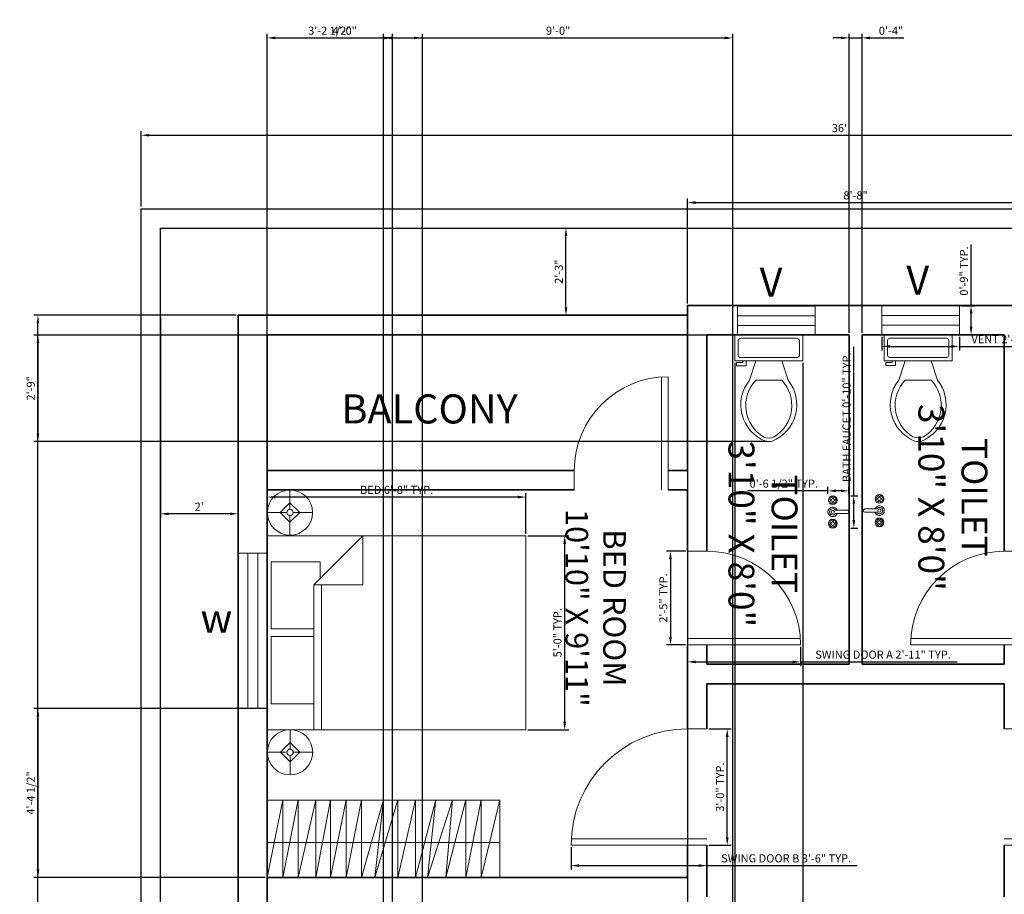
# Model space of a CAD drawing. Units: inches. Extents: x 1879 to 2382, y 1769 to 2461.
# Tile 4 of 5: x 1879 to 2183, y 2190 to 2461. Entities that reach past the tile are written whole.
import ezdxf

# ---------------------------------------------------------------- set-up
doc = ezdxf.new("R2010")
doc.units = ezdxf.units.IN
for name, color, linetype, lineweight in [('A-ANNO-DIMS', 2, 'Continuous', 18), ('A-ANNO-TEXT', 3, 'Continuous', 18), ('A-AREA-IDEN', 7, 'Continuous', 18), ('A-DOOR', 3, 'Continuous', 18), ('A-FLOR-CASE', 8, 'Continuous', 18), ('A-FLOR-FIXT', 9, 'Continuous', 18), ('A-FURN', 9, 'Continuous', 18), ('A-GLAZ', 4, 'Continuous', 18), ('A-WALL', 7, 'Continuous', 35), ('C-PROP', 1, 'Continuous', 25)]:
    doc.layers.add(name, color=color, linetype=linetype, lineweight=lineweight)
doc.styles.get("Standard").update_dxf_attribs({"font": 'arial.ttf'})
doc.dimstyles.new('ISO-25', dxfattribs={"dimtxt": 2.5, "dimasz": 2.5, "dimexe": 1.25, "dimexo": 0.625, "dimtad": 1, "dimlunit": 4, "dimtxsty": 'Standard', "dimcen": 2.5, "dimadec": 0, "dimazin": 0, "dimtfac": 1, "dimtmove": 0, "dimatfit": 3, "dimfxl": 1, "dimarcsym": 0})

# ---------------------------------------------------------------- blocks, each defined once
blk = doc.blocks.new('*D1')
at = {"layer": 'A-ANNO-DIMS', "color": 0, "lineweight": -2, "transparency": 16777216}
for p, q in [((1916.34, 2402.81), (1916.34, 2426.16)), ((1918.84, 2424.91), (2345.84, 2424.91)), ((2348.34, 2402.81), (2348.34, 2426.16))]:
    blk.add_line(p, q, dxfattribs=at)
at = {"layer": 'A-ANNO-DIMS', "color": 0, "transparency": 16777216}
for points in [[(1918.84, 2425.32), (1918.84, 2424.49), (1916.34, 2424.91)], [(2345.84, 2425.32), (2345.84, 2424.49), (2348.34, 2424.91)]]:
    blk.add_solid(points, dxfattribs=at)
at = {"layer": 'Defpoints', "color": 0, "transparency": 16777216}
for p in [(2348.34, 2424.91), (1916.34, 2402.18), (2348.34, 2402.18)]:
    blk.add_point(p, dxfattribs=at)
at = {"layer": 'A-ANNO-DIMS', "color": 0, "transparency": 16777216, "insert": (2132.34, 2426.81), "char_height": 2.5, "attachment_point": 5}
blk.add_mtext("36'", dxfattribs=at)
blk = doc.blocks.new('*U4')
for p, q in [((9.5, -6), (9.5, -2)), ((-10, -8.5), (-8, -8.5)), ((-10, -9.5), (-10, -8.5)), ((-8, -8.5), (-8, -8)), ((-7, -8), (-7, -9.5)), ((-4, -8), (-6, -14)), ((4, -8), (6, -14)), ((-7, -9.5), (-10, -9.5)), ((4, -14), (-4, -14))]:
    blk.add_line(p, q)
blk.add_lwpolyline([(10.5, -8), (10.5, 0), (-10.5, 0), (-10.5, -8)], close=True)
for points in [[(-9.5, -2), (-9.5, -6)], [(8.5, -1), (-8.5, -1)], [(-8.5, -7), (8.5, -7)]]:
    blk.add_lwpolyline(points)
for centre, radius, start, end in [((-8.62, -1.88), 0.884, 81.8699, 188.1301), ((8.62, -1.88), 0.884, 351.8699, 98.1301), ((-8.62, -6.12), 0.884, 171.8699, 278.1301), ((8.62, -6.12), 0.884, 261.8699, 8.1301), ((3.52, -21.58), 12.17, 141.4691, 247.9714), ((4.2, -21.82), 11.33, 136.3677, 238.9468), ((-3.52, -21.58), 12.17, 292.0284, 38.5307), ((-4.2, -21.82), 11.33, 301.053, 43.6321), ((0, -27.88), 4, 245.7318, 294.2682), ((0, -29), 4, 254.8605, 285.1395)]:
    blk.add_arc(centre, radius, start, end)
blk = doc.blocks.new('Bed - Queen')
for p, q in [((0, -80.00003), (0, 0)), ((0, 0), (59.99999, 0)), ((59.99999, 0), (59.99999, -80.00003)), ((7.99999, -1.2), (28.79998, -1.2)), ((7.99999, -14.4), (7.99999, -1.2)), ((28.79998, -1.2), (28.79998, -14.4)), ((31.19999, -1.2), (51.99999, -1.2)), ((31.19999, -14.4), (31.19999, -1.2)), ((51.99999, -1.2), (51.99999, -16.4)), ((0, -14.4), (44.8, -14.4)), ((59.99999, -29.6), (44.8, -14.4)), ((44.8, -14.4), (44.8, -29.6)), ((44.8, -16.8), (0, -16.8)), ((51.99999, -16.4), (46.79936, -16.4)), ((44.8, -29.6), (59.99999, -29.6)), ((59.99999, -80.00003), (0, -80.00003))]:
    blk.add_line(p, q)
blk = doc.blocks.new('Lamp - Table')
for p, q in [((0, 7), (0, 1)), ((-1, 0), (-7, 0)), ((0, 3), (-3, 0)), ((-3, 0), (0, -3)), ((3, 0), (0, 3)), ((0, -3), (3, 0)), ((1, 0), (7, 0)), ((0, -1), (0, -7))]:
    blk.add_line(p, q)
for radius in [7, 1]:
    blk.add_circle((0, 0), radius)
blk = doc.blocks.new('Faucet - Bathroom top')
for p, q in [((-4.107, 0.125), (-4.375, 0.125)), ((-3.75, 0.4788), (-3.75, 0.75)), ((-3.5, 0.482), (-3.5, 0.75)), ((-3.1461, 0.125), (-2.875, 0.125)), ((3.143, 0.125), (2.875, 0.125)), ((3.5, 0.4788), (3.5, 0.75)), ((3.75, 0.482), (3.75, 0.75)), ((4.1039, 0.125), (4.375, 0.125)), ((-4.1039, -0.125), (-4.375, -0.125)), ((-3.75, -0.4821), (-3.75, -0.75)), ((-3.5, -0.4789), (-3.5, -0.75)), ((-3.143, -0.125), (-2.875, -0.125)), ((-0.5, -0.8639), (-0.5, -4.5)), ((0.5, -4.5), (0.5, -0.8631)), ((3.1461, -0.125), (2.875, -0.125)), ((3.5, -0.4821), (3.5, -0.75)), ((3.75, -0.4789), (3.75, -0.75)), ((4.107, -0.125), (4.375, -0.125))]:
    blk.add_line(p, q)
for centre, radius in [((-3.625, 0), 1.375), ((-4.625, 0), 0.2795), ((-3.625, 0), 0.5), ((-3.625, 1), 0.2795), ((-2.625, 0), 0.2795), ((0, 0), 0.5), ((3.625, 0), 1.375), ((2.625, 0), 0.2795), ((3.625, 0), 0.5), ((3.625, 1), 0.2795), ((4.625, 0), 0.2795), ((-3.625, -1), 0.2795), ((3.625, -1), 0.2795)]:
    blk.add_circle(centre, radius)
for centre, radius, start, end in [((-3.625, 0), 1, 105.2407, 164.2093), ((-3.625, 0), 1, 16.44125, 74.07887), ((0, 0), 1.5, 289.6514, 250.3603), ((0, 0), 1, 300.3431, 239.7554), ((3.625, 0), 1, 106.12, 164.0884), ((3.625, 0), 1, 16.23422, 73.90469), ((-3.625, 0), 1, 196.2342, 253.9047), ((-3.625, 0), 1, 286.12, 344.0884), ((3.625, 0), 1, 196.4413, 254.0789), ((3.625, 0), 1, 285.2407, 344.2093), ((0, -4.5), 0.5, 180, 0)]:
    blk.add_arc(centre, radius, start, end)
blk = doc.blocks.new('*D14')
at = {"layer": 'A-ANNO-DIMS', "color": 0, "lineweight": -2, "transparency": 16777216}
for p, q in [((1946.97, 2396.18), (2049.02, 2396.18)), ((2047.77, 2371.68), (2047.77, 2393.68)), ((1946.97, 2369.18), (2049.02, 2369.18))]:
    blk.add_line(p, q, dxfattribs=at)
at = {"layer": 'A-ANNO-DIMS', "color": 0, "transparency": 16777216}
for points in [[(2047.36, 2393.68), (2048.19, 2393.68), (2047.77, 2396.18)], [(2047.36, 2371.68), (2048.19, 2371.68), (2047.77, 2369.18)]]:
    blk.add_solid(points, dxfattribs=at)
at = {"layer": 'Defpoints', "color": 0, "transparency": 16777216}
for p in [(1946.34, 2396.18), (2047.77, 2396.18), (1946.34, 2369.18)]:
    blk.add_point(p, dxfattribs=at)
at = {"layer": 'A-ANNO-DIMS', "color": 0, "transparency": 16777216, "insert": (2045.87, 2382.68), "char_height": 2.5, "attachment_point": 5, "rotation": 90}
blk.add_mtext('2\'-3"', dxfattribs=at)
blk = doc.blocks.new('*D19')
at = {"layer": 'A-ANNO-DIMS', "color": 0, "lineweight": -2, "transparency": 16777216}
for p, q in [((1922.34, 2368.56), (1922.34, 2306.49)), ((1946.34, 2368.56), (1946.34, 2306.49)), ((1943.84, 2307.74), (1924.84, 2307.74))]:
    blk.add_line(p, q, dxfattribs=at)
at = {"layer": 'A-ANNO-DIMS', "color": 0, "transparency": 16777216}
for points in [[(1924.84, 2308.16), (1924.84, 2307.33), (1922.34, 2307.74)], [(1943.84, 2308.16), (1943.84, 2307.33), (1946.34, 2307.74)]]:
    blk.add_solid(points, dxfattribs=at)
at = {"layer": 'Defpoints', "color": 0, "transparency": 16777216}
for p in [(1922.34, 2369.18), (1946.34, 2369.18), (1922.34, 2307.74)]:
    blk.add_point(p, dxfattribs=at)
at = {"layer": 'A-ANNO-DIMS', "color": 0, "transparency": 16777216, "insert": (1934.34, 2309.62), "char_height": 2.5, "attachment_point": 5}
blk.add_mtext("2'", dxfattribs=at)
blk = doc.blocks.new('WN-48x9')
for p, q in [((0, 48), (0, 0)), ((9, 48), (0, 48)), ((3, 48), (3, 0)), ((6, 0), (6, 48)), ((9, 0), (9, 48)), ((0, 0), (9, 0))]:
    blk.add_line(p, q)
blk = doc.blocks.new('VENT-24x9')
for p, q in [((24, 9), (0, 9)), ((0, 9), (0, 0)), ((24, 9), (24, 0)), ((24, 6), (0, 6)), ((0, 3), (24, 3)), ((0, 0), (24, 0))]:
    blk.add_line(p, q)
blk = doc.blocks.new('DR-SWING-29')
for p, q in [((27, 6), (27, 35)), ((29, 6), (29, 35)), ((0, 0), (0, 6)), ((27, 6), (27, 0)), ((29, 6), (29, 0))]:
    blk.add_line(p, q)
blk.add_arc((29, 6), 29, 90, 180)
blk = doc.blocks.new('DR-SWING-36')
for p, q in [((42, 36), (36, 36)), ((36, 2), (0, 2)), ((36, 0), (0, 0)), ((36, 2), (42, 2)), ((36, 0), (42, 0))]:
    blk.add_line(p, q)
blk.add_arc((36, 0), 36, 90, 180)
blk = doc.blocks.new('WARDROBE-HANGERS-72')
for p, q in [((0, 0), (4.89, 24)), ((4.89, 24), (4.89, 0)), ((4.89, 0), (9.67, 24)), ((9.67, 24), (9.67, 0)), ((9.67, 0), (15.08, 24)), ((15.08, 24), (15.08, 0)), ((15.08, 0), (19.6, 24)), ((19.6, 24), (19.6, 0)), ((19.6, 0), (24.51, 24)), ((24.51, 24), (24.51, 0)), ((24.51, 0), (29.16, 24)), ((29.16, 24), (29.16, 0)), ((29.16, 0), (36, 24)), ((36, 24), (33.31, 0)), ((33.31, 0), (40.47, 24)), ((40.47, 24), (40.47, 0)), ((40.47, 0), (45.88, 24)), ((45.88, 24), (45.88, 0)), ((45.88, 0), (52.17, 24)), ((52.17, 24), (49.65, 0)), ((49.65, 0), (57.32, 24)), ((57.32, 24), (55.31, 0)), ((55.31, 0), (61.47, 24)), ((61.47, 24), (61.47, 0)), ((61.47, 0), (66.25, 24)), ((66.25, 24), (66.25, 0)), ((66.25, 0), (72, 24))]:
    blk.add_line(p, q)
blk = doc.blocks.new('*D31')
at = {"layer": 'A-ANNO-DIMS', "color": 0, "lineweight": -2, "transparency": 16777216}
for p, q in [((2085.34, 2266.56), (2085.34, 2260.68)), ((2120.34, 2266.56), (2120.34, 2260.68)), ((2087.84, 2261.93), (2117.84, 2261.93)), ((2120.34, 2261.93), (2168.81, 2261.93))]:
    blk.add_line(p, q, dxfattribs=at)
at = {"layer": 'A-ANNO-DIMS', "color": 0, "transparency": 16777216}
for points in [[(2087.84, 2262.35), (2087.84, 2261.51), (2085.34, 2261.93)], [(2117.84, 2262.35), (2117.84, 2261.51), (2120.34, 2261.93)]]:
    blk.add_solid(points, dxfattribs=at)
at = {"layer": 'Defpoints', "color": 0, "transparency": 16777216}
for p in [(2085.34, 2267.18), (2120.34, 2267.18), (2120.34, 2261.93)]:
    blk.add_point(p, dxfattribs=at)
at = {"layer": 'A-ANNO-DIMS', "color": 0, "transparency": 16777216, "insert": (2145.83, 2263.85), "char_height": 2.5, "attachment_point": 5}
blk.add_mtext('SWING DOOR A 2\'-11" TYP.', dxfattribs=at)
blk = doc.blocks.new('*D32')
at = {"layer": 'A-ANNO-DIMS', "color": 0, "lineweight": -2, "transparency": 16777216}
for p, q in [((2084.72, 2296.18), (2078.84, 2296.18)), ((2080.09, 2293.68), (2080.09, 2269.68)), ((2084.72, 2267.18), (2078.84, 2267.18))]:
    blk.add_line(p, q, dxfattribs=at)
at = {"layer": 'A-ANNO-DIMS', "color": 0, "transparency": 16777216}
for points in [[(2079.67, 2293.68), (2080.51, 2293.68), (2080.09, 2296.18)], [(2079.67, 2269.68), (2080.51, 2269.68), (2080.09, 2267.18)]]:
    blk.add_solid(points, dxfattribs=at)
at = {"layer": 'Defpoints', "color": 0, "transparency": 16777216}
for p in [(2085.34, 2296.18), (2080.09, 2267.18), (2085.34, 2267.18)]:
    blk.add_point(p, dxfattribs=at)
at = {"layer": 'A-ANNO-DIMS', "color": 0, "transparency": 16777216, "insert": (2078.19, 2281.68), "char_height": 2.5, "attachment_point": 5, "rotation": 90}
blk.add_mtext('2\'-5" TYP.', dxfattribs=at)
blk = doc.blocks.new('*D33')
at = {"layer": 'A-ANNO-DIMS', "color": 0, "lineweight": -2, "transparency": 16777216}
for p, q in [((2049.34, 2204.56), (2049.34, 2197.63)), ((2091.34, 2204.56), (2091.34, 2197.63)), ((2051.84, 2198.88), (2088.84, 2198.88)), ((2091.34, 2198.88), (2137.87, 2198.88))]:
    blk.add_line(p, q, dxfattribs=at)
at = {"layer": 'A-ANNO-DIMS', "color": 0, "transparency": 16777216}
for points in [[(2051.84, 2199.3), (2051.84, 2198.46), (2049.34, 2198.88)], [(2088.84, 2199.3), (2088.84, 2198.46), (2091.34, 2198.88)]]:
    blk.add_solid(points, dxfattribs=at)
at = {"layer": 'Defpoints', "color": 0, "transparency": 16777216}
for p in [(2049.34, 2205.18), (2091.34, 2205.18), (2091.34, 2198.88)]:
    blk.add_point(p, dxfattribs=at)
at = {"layer": 'A-ANNO-DIMS', "color": 0, "transparency": 16777216, "insert": (2115.86, 2200.8), "char_height": 2.5, "attachment_point": 5}
blk.add_mtext('SWING DOOR B 3\'-6" TYP.', dxfattribs=at)
blk = doc.blocks.new('*D34')
at = {"layer": 'A-ANNO-DIMS', "color": 0, "lineweight": -2, "transparency": 16777216}
for p, q in [((2091.97, 2241.18), (2098.89, 2241.18)), ((2097.64, 2207.68), (2097.64, 2238.68)), ((2091.97, 2205.18), (2098.89, 2205.18))]:
    blk.add_line(p, q, dxfattribs=at)
at = {"layer": 'A-ANNO-DIMS', "color": 0, "transparency": 16777216}
for points in [[(2097.22, 2238.68), (2098.06, 2238.68), (2097.64, 2241.18)], [(2097.22, 2207.68), (2098.06, 2207.68), (2097.64, 2205.18)]]:
    blk.add_solid(points, dxfattribs=at)
at = {"layer": 'Defpoints', "color": 0, "transparency": 16777216}
for p in [(2091.34, 2241.18), (2097.64, 2241.18), (2091.34, 2205.18)]:
    blk.add_point(p, dxfattribs=at)
at = {"layer": 'A-ANNO-DIMS', "color": 0, "transparency": 16777216, "insert": (2095.74, 2223.18), "char_height": 2.5, "attachment_point": 5, "rotation": 90}
blk.add_mtext('3\'-0" TYP.', dxfattribs=at)
blk = doc.blocks.new('*D35')
at = {"layer": 'A-ANNO-DIMS', "color": 0, "lineweight": -2, "transparency": 16777216}
for p, q in [((2145.46, 2362.53), (2145.46, 2358.3)), ((2169.46, 2362.53), (2169.46, 2358.3)), ((2147.96, 2359.55), (2166.96, 2359.55)), ((2169.46, 2359.55), (2198.87, 2359.55))]:
    blk.add_line(p, q, dxfattribs=at)
at = {"layer": 'A-ANNO-DIMS', "color": 0, "transparency": 16777216}
for points in [[(2147.96, 2359.97), (2147.96, 2359.14), (2145.46, 2359.55)], [(2166.96, 2359.97), (2166.96, 2359.14), (2169.46, 2359.55)]]:
    blk.add_solid(points, dxfattribs=at)
at = {"layer": 'Defpoints', "color": 0, "transparency": 16777216}
for p in [(2145.46, 2363.15), (2169.46, 2363.15), (2169.46, 2359.55)]:
    blk.add_point(p, dxfattribs=at)
at = {"layer": 'A-ANNO-DIMS', "color": 0, "transparency": 16777216, "insert": (2185.41, 2361.45), "char_height": 2.5, "attachment_point": 5}
blk.add_mtext('VENT 2\'-0" TYP.', dxfattribs=at)
blk = doc.blocks.new('*D36')
at = {"layer": 'A-ANNO-DIMS', "color": 0, "lineweight": -2, "transparency": 16777216}
for p, q in [((2173.06, 2372.15), (2173.06, 2391.14)), ((2170.09, 2372.15), (2174.31, 2372.15)), ((2173.06, 2365.65), (2173.06, 2369.65)), ((2170.09, 2363.15), (2174.31, 2363.15))]:
    blk.add_line(p, q, dxfattribs=at)
at = {"layer": 'A-ANNO-DIMS', "color": 0, "transparency": 16777216}
for points in [[(2172.65, 2369.65), (2173.48, 2369.65), (2173.06, 2372.15)], [(2172.65, 2365.65), (2173.48, 2365.65), (2173.06, 2363.15)]]:
    blk.add_solid(points, dxfattribs=at)
at = {"layer": 'Defpoints', "color": 0, "transparency": 16777216}
for p in [(2169.46, 2372.15), (2173.06, 2372.15), (2169.46, 2363.15)]:
    blk.add_point(p, dxfattribs=at)
at = {"layer": 'A-ANNO-DIMS', "color": 0, "transparency": 16777216, "insert": (2171.16, 2382.9), "char_height": 2.5, "attachment_point": 5, "rotation": 90}
blk.add_mtext('0\'-9" TYP.', dxfattribs=at)
blk = doc.blocks.new('*D39')
at = {"layer": 'A-ANNO-DIMS', "color": 0, "lineweight": -2, "transparency": 16777216}
for p, q in [((1955.37, 2301.56), (1955.37, 2314.19)), ((2032.87, 2312.94), (1957.87, 2312.94)), ((2035.37, 2301.56), (2035.37, 2314.19))]:
    blk.add_line(p, q, dxfattribs=at)
at = {"layer": 'A-ANNO-DIMS', "color": 0, "transparency": 16777216}
for points in [[(1957.87, 2313.36), (1957.87, 2312.52), (1955.37, 2312.94)], [(2032.87, 2313.36), (2032.87, 2312.52), (2035.37, 2312.94)]]:
    blk.add_solid(points, dxfattribs=at)
at = {"layer": 'Defpoints', "color": 0, "transparency": 16777216}
for p in [(1955.37, 2312.94), (1955.37, 2300.94), (2035.37, 2300.94)]:
    blk.add_point(p, dxfattribs=at)
at = {"layer": 'A-ANNO-DIMS', "color": 0, "transparency": 16777216, "insert": (1995.37, 2314.84), "char_height": 2.5, "attachment_point": 5}
blk.add_mtext('BED 6\'-8" TYP.', dxfattribs=at)
blk = doc.blocks.new('*D40')
at = {"layer": 'A-ANNO-DIMS', "color": 0, "lineweight": -2, "transparency": 16777216}
for p, q in [((2035.99, 2300.94), (2048.62, 2300.94)), ((2047.37, 2243.44), (2047.37, 2298.44)), ((2035.99, 2240.94), (2048.62, 2240.94))]:
    blk.add_line(p, q, dxfattribs=at)
at = {"layer": 'A-ANNO-DIMS', "color": 0, "transparency": 16777216}
for points in [[(2046.95, 2298.44), (2047.79, 2298.44), (2047.37, 2300.94)], [(2046.95, 2243.44), (2047.79, 2243.44), (2047.37, 2240.94)]]:
    blk.add_solid(points, dxfattribs=at)
at = {"layer": 'Defpoints', "color": 0, "transparency": 16777216}
for p in [(2035.37, 2300.94), (2047.37, 2300.94), (2035.37, 2240.94)]:
    blk.add_point(p, dxfattribs=at)
at = {"layer": 'A-ANNO-DIMS', "color": 0, "transparency": 16777216, "insert": (2045.47, 2270.94), "char_height": 2.5, "attachment_point": 5, "rotation": 90}
blk.add_mtext('5\'-0" TYP.', dxfattribs=at)
blk = doc.blocks.new('*D43')
at = {"layer": 'A-ANNO-DIMS', "color": 0, "lineweight": -2, "transparency": 16777216}
for p, q in [((2136.79, 2313.35), (2136.79, 2359.4)), ((2135.92, 2313.35), (2138.04, 2313.35)), ((2136.79, 2305.85), (2136.79, 2310.85)), ((2135.92, 2303.35), (2138.04, 2303.35))]:
    blk.add_line(p, q, dxfattribs=at)
at = {"layer": 'A-ANNO-DIMS', "color": 0, "transparency": 16777216}
for points in [[(2136.37, 2310.85), (2137.21, 2310.85), (2136.79, 2313.35)], [(2136.37, 2305.85), (2137.21, 2305.85), (2136.79, 2303.35)]]:
    blk.add_solid(points, dxfattribs=at)
at = {"layer": 'Defpoints', "color": 0, "transparency": 16777216}
for p in [(2135.29, 2313.35), (2136.79, 2313.35), (2135.29, 2303.35)]:
    blk.add_point(p, dxfattribs=at)
at = {"layer": 'A-ANNO-DIMS', "color": 0, "transparency": 16777216, "insert": (2134.87, 2337.63), "char_height": 2.5, "attachment_point": 5, "rotation": 90}
blk.add_mtext('BATH FAUCET 0\'-10" TYP.', dxfattribs=at)
blk = doc.blocks.new('*D44')
at = {"layer": 'A-ANNO-DIMS', "color": 0, "lineweight": -2, "transparency": 16777216}
for p, q in [((2128.79, 2314.85), (2103.98, 2314.85)), ((2128.79, 2313.98), (2128.79, 2316.1)), ((2132.79, 2314.85), (2131.29, 2314.85)), ((2135.29, 2313.98), (2135.29, 2316.1))]:
    blk.add_line(p, q, dxfattribs=at)
at = {"layer": 'A-ANNO-DIMS', "color": 0, "transparency": 16777216}
for points in [[(2131.29, 2315.27), (2131.29, 2314.44), (2128.79, 2314.85)], [(2132.79, 2315.27), (2132.79, 2314.44), (2135.29, 2314.85)]]:
    blk.add_solid(points, dxfattribs=at)
at = {"layer": 'Defpoints', "color": 0, "transparency": 16777216}
for p in [(2128.79, 2314.85), (2128.79, 2313.35), (2135.29, 2313.35)]:
    blk.add_point(p, dxfattribs=at)
at = {"layer": 'A-ANNO-DIMS', "color": 0, "transparency": 16777216, "insert": (2115.13, 2316.77), "char_height": 2.5, "attachment_point": 5}
blk.add_mtext('0\'-6 1/2" TYP.', dxfattribs=at)
blk = doc.blocks.new('*D56')
at = {"layer": 'A-ANNO-DIMS', "color": 0, "lineweight": -2, "transparency": 16777216}
for p, q in [((1945.72, 2369.18), (1883.19, 2369.18)), ((1884.44, 1810.68), (1884.44, 2366.68)), ((1945.72, 1808.18), (1883.19, 1808.18))]:
    blk.add_line(p, q, dxfattribs=at)
at = {"layer": 'A-ANNO-DIMS', "color": 0, "transparency": 16777216}
for points in [[(1884.02, 2366.68), (1884.86, 2366.68), (1884.44, 2369.18)], [(1884.02, 1810.68), (1884.86, 1810.68), (1884.44, 1808.18)]]:
    blk.add_solid(points, dxfattribs=at)
at = {"layer": 'Defpoints', "color": 0, "transparency": 16777216}
for p in [(1884.44, 2369.18), (1946.34, 2369.18), (1946.34, 1808.18)]:
    blk.add_point(p, dxfattribs=at)
at = {"layer": 'A-ANNO-DIMS', "color": 0, "transparency": 16777216, "insert": (1882.54, 2088.68), "char_height": 2.5, "attachment_point": 5, "rotation": 90}
blk.add_mtext('46\'-9"', dxfattribs=at)
blk = doc.blocks.new('*D61')
at = {"layer": 'A-ANNO-DIMS', "color": 0, "lineweight": -2, "transparency": 16777216}
for p, q in [((1955.34, 2015.81), (1955.34, 2456.28)), ((1957.84, 2455.03), (2000.84, 2455.03)), ((2003.34, 2015.81), (2003.34, 2456.28))]:
    blk.add_line(p, q, dxfattribs=at)
at = {"layer": 'A-ANNO-DIMS', "color": 0, "transparency": 16777216}
for points in [[(1957.84, 2455.44), (1957.84, 2454.61), (1955.34, 2455.03)], [(2000.84, 2455.44), (2000.84, 2454.61), (2003.34, 2455.03)]]:
    blk.add_solid(points, dxfattribs=at)
at = {"layer": 'Defpoints', "color": 0, "transparency": 16777216}
for p in [(2003.34, 2455.03), (1955.34, 2015.18), (2003.34, 2015.18)]:
    blk.add_point(p, dxfattribs=at)
at = {"layer": 'A-ANNO-DIMS', "color": 0, "transparency": 16777216, "insert": (1979.34, 2456.93), "char_height": 2.5, "attachment_point": 5}
blk.add_mtext('4\'-0"', dxfattribs=at)
blk = doc.blocks.new('*D62')
at = {"layer": 'A-ANNO-DIMS', "color": 0, "lineweight": -2, "transparency": 16777216}
for p, q in [((2099.99, 2354.46), (2099.99, 1769.03)), ((2120.99, 2354.46), (2120.99, 1769.03)), ((2102.49, 1770.28), (2118.49, 1770.28))]:
    blk.add_line(p, q, dxfattribs=at)
at = {"layer": 'A-ANNO-DIMS', "color": 0, "transparency": 16777216}
for points in [[(2102.49, 1770.7), (2102.49, 1769.86), (2099.99, 1770.28)], [(2118.49, 1770.7), (2118.49, 1769.86), (2120.99, 1770.28)]]:
    blk.add_solid(points, dxfattribs=at)
at = {"layer": 'Defpoints', "color": 0, "transparency": 16777216}
for p in [(2099.99, 2355.08), (2120.99, 2355.08), (2120.99, 1770.28)]:
    blk.add_point(p, dxfattribs=at)
at = {"layer": 'A-ANNO-DIMS', "color": 0, "transparency": 16777216, "insert": (2110.49, 1772.18), "char_height": 2.5, "attachment_point": 5}
blk.add_mtext('1\'-9"', dxfattribs=at)
blk = doc.blocks.new('*D63')
at = {"layer": 'A-ANNO-DIMS', "color": 0, "lineweight": -2, "transparency": 16777216}
for p, q in [((2099.36, 2363.08), (1883.19, 2363.08)), ((1884.44, 2360.58), (1884.44, 2332.58)), ((2109.86, 2330.08), (1883.19, 2330.08))]:
    blk.add_line(p, q, dxfattribs=at)
at = {"layer": 'A-ANNO-DIMS', "color": 0, "transparency": 16777216}
for points in [[(1884.02, 2360.58), (1884.86, 2360.58), (1884.44, 2363.08)], [(1884.02, 2332.58), (1884.86, 2332.58), (1884.44, 2330.08)]]:
    blk.add_solid(points, dxfattribs=at)
at = {"layer": 'Defpoints', "color": 0, "transparency": 16777216}
for p in [(2099.99, 2363.08), (1884.44, 2330.08), (2110.49, 2330.08)]:
    blk.add_point(p, dxfattribs=at)
at = {"layer": 'A-ANNO-DIMS', "color": 0, "transparency": 16777216, "insert": (1882.54, 2346.58), "char_height": 2.5, "attachment_point": 5, "rotation": 90}
blk.add_mtext('2\'-9"', dxfattribs=at)
blk = doc.blocks.new('*D64')
at = {"layer": 'A-ANNO-DIMS', "color": 0, "lineweight": -2, "transparency": 16777216}
for p, q in [((2132.84, 2455.03), (2130.34, 2455.03)), ((2135.34, 2363.81), (2135.34, 2456.28)), ((2135.34, 2455.03), (2139.34, 2455.03)), ((2139.34, 2363.81), (2139.34, 2456.28)), ((2141.84, 2455.03), (2152.24, 2455.03))]:
    blk.add_line(p, q, dxfattribs=at)
at = {"layer": 'A-ANNO-DIMS', "color": 0, "transparency": 16777216}
for points in [[(2132.84, 2455.44), (2132.84, 2454.61), (2135.34, 2455.03)], [(2141.84, 2455.44), (2141.84, 2454.61), (2139.34, 2455.03)]]:
    blk.add_solid(points, dxfattribs=at)
at = {"layer": 'Defpoints', "color": 0, "transparency": 16777216}
for p in [(2139.34, 2455.03), (2135.34, 2363.18), (2139.34, 2363.18)]:
    blk.add_point(p, dxfattribs=at)
at = {"layer": 'A-ANNO-DIMS', "color": 0, "transparency": 16777216, "insert": (2148.29, 2456.93), "char_height": 2.5, "attachment_point": 5}
blk.add_mtext('0\'-4"', dxfattribs=at)
blk = doc.blocks.new('*D65')
at = {"layer": 'A-ANNO-DIMS', "color": 0, "lineweight": -2, "transparency": 16777216}
for p, q in [((1991.34, 1850.81), (1991.34, 2456.28)), ((1993.84, 2455.03), (2096.84, 2455.03)), ((2099.34, 1850.81), (2099.34, 2456.28))]:
    blk.add_line(p, q, dxfattribs=at)
at = {"layer": 'A-ANNO-DIMS', "color": 0, "transparency": 16777216}
for points in [[(1993.84, 2455.44), (1993.84, 2454.61), (1991.34, 2455.03)], [(2096.84, 2455.44), (2096.84, 2454.61), (2099.34, 2455.03)]]:
    blk.add_solid(points, dxfattribs=at)
at = {"layer": 'Defpoints', "color": 0, "transparency": 16777216}
for p in [(2099.34, 2455.03), (1991.34, 1850.18), (2099.34, 1850.18)]:
    blk.add_point(p, dxfattribs=at)
at = {"layer": 'A-ANNO-DIMS', "color": 0, "transparency": 16777216, "insert": (2045.34, 2456.93), "char_height": 2.5, "attachment_point": 5}
blk.add_mtext('9\'-0"', dxfattribs=at)
blk = doc.blocks.new('*D67')
at = {"layer": 'A-ANNO-DIMS', "color": 0, "lineweight": -2, "transparency": 16777216}
for p, q in [((1955.34, 1901.81), (1955.34, 2456.28)), ((1957.84, 2455.03), (1991.58, 2455.03)), ((1994.08, 1901.81), (1994.08, 2456.28))]:
    blk.add_line(p, q, dxfattribs=at)
at = {"layer": 'A-ANNO-DIMS', "color": 0, "transparency": 16777216}
for points in [[(1957.84, 2455.44), (1957.84, 2454.61), (1955.34, 2455.03)], [(1991.58, 2455.44), (1991.58, 2454.61), (1994.08, 2455.03)]]:
    blk.add_solid(points, dxfattribs=at)
at = {"layer": 'Defpoints', "color": 0, "transparency": 16777216}
for p in [(1994.08, 2455.03), (1955.34, 1901.18), (1994.08, 1901.18)]:
    blk.add_point(p, dxfattribs=at)
at = {"layer": 'A-ANNO-DIMS', "color": 0, "transparency": 16777216, "insert": (1974.71, 2456.95), "char_height": 2.5, "attachment_point": 5}
blk.add_mtext('3\'-2 1/2"', dxfattribs=at)
blk = doc.blocks.new('*D71')
at = {"layer": 'A-ANNO-DIMS', "color": 0, "lineweight": -2, "transparency": 16777216}
for p, q in [((1955.34, 2362.56), (1955.34, 1769.03)), ((2085.34, 2362.56), (2085.34, 1769.03)), ((1957.84, 1770.28), (2082.84, 1770.28))]:
    blk.add_line(p, q, dxfattribs=at)
at = {"layer": 'A-ANNO-DIMS', "color": 0, "transparency": 16777216}
for points in [[(1957.84, 1770.7), (1957.84, 1769.86), (1955.34, 1770.28)], [(2082.84, 1770.7), (2082.84, 1769.86), (2085.34, 1770.28)]]:
    blk.add_solid(points, dxfattribs=at)
at = {"layer": 'Defpoints', "color": 0, "transparency": 16777216}
for p in [(1955.34, 2363.18), (2085.34, 2363.18), (2085.34, 1770.28)]:
    blk.add_point(p, dxfattribs=at)
at = {"layer": 'A-ANNO-DIMS', "color": 0, "transparency": 16777216, "insert": (2020.34, 1772.18), "char_height": 2.5, "attachment_point": 5}
blk.add_mtext('10\'-10"', dxfattribs=at)
blk = doc.blocks.new('*D73')
at = {"layer": 'A-ANNO-DIMS', "color": 0, "lineweight": -2, "transparency": 16777216}
for p, q in [((1954.78, 2247.54), (1883.19, 2247.54)), ((1884.44, 2245.04), (1884.44, 2197.68)), ((1954.72, 2195.18), (1883.19, 2195.18))]:
    blk.add_line(p, q, dxfattribs=at)
at = {"layer": 'A-ANNO-DIMS', "color": 0, "transparency": 16777216}
for points in [[(1884.02, 2245.04), (1884.86, 2245.04), (1884.44, 2247.54)], [(1884.02, 2197.68), (1884.86, 2197.68), (1884.44, 2195.18)]]:
    blk.add_solid(points, dxfattribs=at)
at = {"layer": 'Defpoints', "color": 0, "transparency": 16777216}
for p in [(1955.4, 2247.54), (1884.44, 2195.18), (1955.34, 2195.18)]:
    blk.add_point(p, dxfattribs=at)
at = {"layer": 'A-ANNO-DIMS', "color": 0, "transparency": 16777216, "insert": (1882.52, 2221.36), "char_height": 2.5, "attachment_point": 5, "rotation": 90}
blk.add_mtext('4\'-4 1/2"', dxfattribs=at)
blk = doc.blocks.new('*D78')
at = {"layer": 'A-ANNO-DIMS', "color": 0, "lineweight": -2, "transparency": 16777216}
for p, q in [((2085.34, 2372.81), (2085.33, 2405.33)), ((2087.84, 2404.08), (2186.84, 2404.1)), ((2189.34, 2372.83), (2189.33, 2405.35))]:
    blk.add_line(p, q, dxfattribs=at)
at = {"layer": 'A-ANNO-DIMS', "color": 0, "transparency": 16777216}
for points in [[(2087.84, 2404.5), (2087.84, 2403.66), (2085.34, 2404.08)], [(2186.84, 2404.52), (2186.84, 2403.68), (2189.34, 2404.1)]]:
    blk.add_solid(points, dxfattribs=at)
at = {"layer": 'Defpoints', "color": 0, "transparency": 16777216}
for p in [(2189.34, 2404.1), (2085.34, 2372.18), (2189.34, 2372.2)]:
    blk.add_point(p, dxfattribs=at)
at = {"layer": 'A-ANNO-DIMS', "color": 0, "transparency": 16777216, "insert": (2137.33, 2405.99), "char_height": 2.5, "attachment_point": 5, "rotation": 0.0111}
blk.add_mtext('8\'-8"', dxfattribs=at)

msp = doc.modelspace()

# ---------------------------------------------------------------- linework, layer by layer
at = {"layer": 'A-FLOR-CASE'}
for p, q in [((1955.341, 2195.18), (1955.341, 2219.18)), ((1955.341, 2219.18), (2027.341, 2219.18)), ((2027.341, 2219.18), (2027.341, 2195.18)), ((2027.341, 2206.006), (1955.341, 2206.006))]:
    msp.add_line(p, q, dxfattribs=at)
at = {"layer": 'A-WALL'}
for p, q in [((2085.341, 2363.18), (2085.341, 2372.181)), ((2085.341, 2372.181), (2092.668, 2372.18)), ((2091.341, 2372.18), (2135.341, 2372.18)), ((2139.341, 2372.18), (2135.341, 2372.18)), ((2139.341, 2372.18), (2183.341, 2372.18)), ((2189.341, 2372.201), (2183.341, 2372.18)), ((1946.341, 2135.18), (1946.341, 2369.18)), ((1955.341, 2369.18), (1946.341, 2369.18)), ((1946.341, 2369.18), (1946.341, 2369.18)), ((1955.341, 2369.18), (2085.341, 2369.18)), ((1955.341, 2363.18), (2085.341, 2363.18)), ((1955.341, 2321.18), (1955.341, 2363.18)), ((2085.341, 2321.18), (2085.341, 2363.18)), ((2091.341, 2363.18), (2135.341, 2363.18)), ((2091.341, 2296.18), (2091.341, 2363.18)), ((2135.341, 2363.18), (2135.341, 2261.18)), ((2139.341, 2261.18), (2139.341, 2363.18)), ((2139.341, 2363.18), (2183.341, 2363.18)), ((2183.341, 2363.18), (2183.341, 2296.18)), ((1955.341, 2321.18), (2050.341, 2321.18)), ((2085.341, 2321.18), (2079.341, 2321.18)), ((2079.341, 2321.18), (2085.341, 2321.18)), ((1955.341, 2315.18), (2050.341, 2315.18)), ((1955.341, 2195.18), (1955.341, 2315.18)), ((2079.341, 2315.18), (2085.341, 2315.18)), ((2085.341, 2296.18), (2085.341, 2315.18)), ((2085.341, 2241.18), (2085.341, 2267.18)), ((2091.341, 2261.18), (2091.341, 2267.18)), ((2091.341, 2261.18), (2091.341, 2267.18)), ((2183.341, 2261.18), (2183.341, 2267.18)), ((2183.341, 2267.18), (2183.341, 2261.18)), ((2091.341, 2261.18), (2135.341, 2261.18)), ((2139.341, 2261.18), (2183.341, 2261.18)), ((2091.341, 2255.18), (2183.341, 2255.18)), ((2091.341, 2241.18), (2091.341, 2255.18)), ((2183.341, 2255.18), (2183.341, 2241.18)), ((2085.341, 2195.18), (2085.341, 2205.18)), ((2085.341, 2195.18), (2085.341, 2205.18)), ((2091.341, 2189.18), (2091.341, 2205.18)), ((2183.341, 2205.18), (2183.341, 2189.18)), ((1955.341, 2195.18), (2085.341, 2195.18))]:
    msp.add_line(p, q, dxfattribs=at)
at = {"layer": 'C-PROP'}
for p, q in [((1916.341, 2402.18), (2348.341, 2402.18)), ((1916.341, 1802.18), (1916.341, 2402.18)), ((1922.341, 1808.18), (1922.341, 2396.18)), ((1922.341, 2396.18), (2342.341, 2396.18))]:
    msp.add_line(p, q, dxfattribs=at)

# ---------------------------------------------------------------- block references
at = {"layer": 'A-DOOR'}
for name, p in [('DR-SWING-29', (2050.341, 2315.18)), ('DR-SWING-36', (2049.341, 2205.18))]:
    msp.add_blockref(name, p, dxfattribs=at)
at = {"layer": 'A-DOOR', "rotation": 269.9999999999977}
msp.add_blockref('DR-SWING-29', (2085.341, 2296.18), dxfattribs=at)
at = {"layer": 'A-DOOR', "extrusion": (0, 0, -1), "zscale": -1, "rotation": 269.9999999999997}
msp.add_blockref('DR-SWING-29', (-2189.341, 2296.18), dxfattribs=at)
at = {"layer": 'A-DOOR', "extrusion": (0, 0, -1), "zscale": -1}
msp.add_blockref('DR-SWING-36', (-2225.341, 2205.18), dxfattribs=at)
at = {"layer": 'A-FLOR-CASE'}
msp.add_blockref('WARDROBE-HANGERS-72', (1955.308, 2195.234), dxfattribs=at)
at = {"layer": 'A-FLOR-FIXT'}
for p in [(2110.487, 2363.082), (2156.704, 2363.128)]:
    msp.add_blockref('*U4', p, dxfattribs=at)
for p, rotation in [((2130.291, 2308.354), 90), ((2144.727, 2308.752), 270)]:
    msp.add_blockref('Faucet - Bathroom top', p, dxfattribs=dict(at, rotation=rotation))
at = {"layer": 'A-FURN'}
for p in [(1962.403, 2308.148), (1962.416, 2233.946)]:
    msp.add_blockref('Lamp - Table', p, dxfattribs=at)
at = {"layer": 'A-FURN', "rotation": 90}
msp.add_blockref('Bed - Queen', (1955.369, 2240.938), dxfattribs=at)
at = {"layer": 'A-GLAZ'}
for p in [(2100.825, 2363.037), (2145.463, 2363.153)]:
    msp.add_blockref('VENT-24x9', p, dxfattribs=at)
at = {"layer": 'A-GLAZ', "rotation": 180}
msp.add_blockref('WN-48x9', (1955.404, 2295.537), dxfattribs=at)

# ---------------------------------------------------------------- texts
at = {"layer": 'A-ANNO-TEXT', "char_height": 9, "attachment_point": 1}
for s, insert in [('\\pxqc;V', (2055.069, 2383.962)), ('\\pxqc;V', (2100.459, 2384.575)), ('\\pxqc;w', (1883.533, 2279.942))]:
    msp.add_mtext_dynamic_manual_height_columns(s, width=112.22887, gutter_width=12.5, heights=[0], dxfattribs=dict(at, insert=insert))
at = {"layer": 'A-AREA-IDEN', "insert": (1978.303, 2344.713), "char_height": 9, "attachment_point": 1}
msp.add_mtext_dynamic_manual_height_columns('BALCONY', width=86.90732, gutter_width=12.5, heights=[0], dxfattribs=at)
at = {"layer": 'A-AREA-IDEN', "attachment_point": 1, "rotation": 270}
for s, width, insert, char_height in [('\\pxqc;TOILET^J3\'10" X 8\'0"', 61.67119, (2178.11, 2343.68), 8), ('\\pxqc;TOILET^J3\'10" X 8\'0"', 61.67119, (2119.369, 2332.405), 8), ('\\pxqc;BED ROOM\\P10\'10" X 9\'11"', 92.15185, (2066.286, 2324.738), 7)]:
    msp.add_mtext_dynamic_manual_height_columns(s, width=width, gutter_width=12.5, heights=[0], dxfattribs=dict(at, insert=insert, char_height=char_height))

# ---------------------------------------------------------------- dimensions: what is measured, and where the dimension line sits
at = {"layer": 'A-ANNO-DIMS'}
for base, p1, p2, override, picture, middle in [((1994.083, 2455.028), (1955.341, 1901.18), (1994.083, 1901.18), {"dimdec": 1, "dimlfac": 1, "dimrnd": 0, "dimzin": 1, "dimdsep": 46, "dimlunit": 4, "dimfrac": 2}, '*D67', (1974.712, 2456.946)), ((2003.341, 2455.028), (1955.341, 2015.18), (2003.341, 2015.18), {"dimdec": 1, "dimlfac": 1, "dimrnd": 0, "dimzin": 1, "dimdsep": 46, "dimlunit": 4, "dimfrac": 2}, '*D61', (1979.341, 2456.929)), ((2099.341, 2455.028), (1991.341, 1850.18), (2099.341, 1850.18), {"dimdec": 1, "dimlfac": 1, "dimrnd": 0, "dimzin": 1, "dimdsep": 46, "dimlunit": 4, "dimfrac": 2}, '*D65', (2045.341, 2456.929)), ((2139.341, 2455.028), (2135.341, 2363.18), (2139.341, 2363.18), {"dimdec": 1, "dimlfac": 1, "dimrnd": 0, "dimzin": 1, "dimdsep": 46, "dimlunit": 4, "dimfrac": 2}, '*D64', (2148.289, 2456.929)), ((2348.341, 2424.907), (1916.341, 2402.18), (2348.341, 2402.18), {"dimclrd": 0, "dimclre": 0, "dimclrt": 0}, '*D1', (2132.341, 2426.81)), ((1922.341, 2307.743), (1946.341, 2369.18), (1922.341, 2369.18), {"dimclrd": 0, "dimclre": 0, "dimclrt": 0}, '*D19', (1934.341, 2309.624)), ((2085.341, 1770.28), (1955.341, 2363.18), (2085.341, 2363.18), {"dimdec": 1, "dimlfac": 1, "dimrnd": 0, "dimzin": 1, "dimdsep": 46, "dimlunit": 4, "dimfrac": 2}, '*D71', (2020.341, 1772.182)), ((2120.987, 1770.28), (2099.987, 2355.082), (2120.987, 2355.082), {"dimdec": 1, "dimlfac": 1, "dimrnd": 0, "dimzin": 1, "dimdsep": 46, "dimlunit": 4, "dimfrac": 2}, '*D62', (2110.487, 1772.182))]:
    dim = msp.add_linear_dim(base=base, p1=p1, p2=p2, dimstyle='ISO-25', override=override, dxfattribs=at)
    dim.commit()
    dim.dimension.update_dxf_attribs({"geometry": picture, "text_midpoint": middle})
for base, p1, p2, angle, override, picture, middle in [((2189.335, 2404.101), (2085.341, 2372.181), (2189.341, 2372.201), 0.01114, {"dimdec": 1, "dimlfac": 1, "dimrnd": 0, "dimzin": 1, "dimdsep": 46, "dimlunit": 4, "dimfrac": 2}, '*D78', (2137.335, 2405.992)), ((2047.774, 2396.18), (1946.341, 2369.18), (1946.341, 2396.18), 90, {"dimclrd": 0, "dimclre": 0, "dimclrt": 0}, '*D14', (2045.872, 2382.68)), ((1884.441, 2369.18), (1946.341, 1808.18), (1946.341, 2369.18), 90, {"dimdec": 1, "dimlfac": 1, "dimrnd": 0, "dimzin": 1, "dimdsep": 46, "dimlunit": 4, "dimfrac": 2}, '*D56', (1882.54, 2088.68)), ((1884.441, 2330.082), (2099.987, 2363.082), (2110.487, 2330.082), 90, {"dimdec": 1, "dimlfac": 1, "dimrnd": 0, "dimzin": 1, "dimdsep": 46, "dimlunit": 4, "dimfrac": 2}, '*D63', (1882.54, 2346.582)), ((1884.441, 2195.18), (1955.404, 2247.537), (1955.341, 2195.18), 90, {"dimdec": 1, "dimlfac": 1, "dimrnd": 0, "dimzin": 1, "dimdsep": 46, "dimlunit": 4, "dimfrac": 2}, '*D73', (1882.524, 2221.359))]:
    dim = msp.add_linear_dim(base=base, p1=p1, p2=p2, angle=angle, dimstyle='ISO-25', override=override, dxfattribs=at)
    dim.commit()
    dim.dimension.update_dxf_attribs({"geometry": picture, "text_midpoint": middle})
for base, p1, p2, angle, text, picture, middle in [((2173.063, 2372.153), (2169.463, 2363.153), (2169.463, 2372.153), 90, '<> TYP.', '*D36', (2171.161, 2382.897)), ((2136.791, 2313.354), (2135.291, 2303.354), (2135.291, 2313.354), 90, 'BATH FAUCET <> TYP.', '*D43', (2134.873, 2337.626)), ((1955.369, 2312.938), (2035.369, 2300.938), (1955.369, 2300.938), 180, 'BED <> TYP.', '*D39', (1995.369, 2314.84)), ((2128.791, 2314.854), (2135.291, 2313.354), (2128.791, 2313.354), 180, '<> TYP.', '*D44', (2115.134, 2316.771)), ((2047.369, 2300.938), (2035.369, 2240.938), (2035.369, 2300.938), 90, '<> TYP.', '*D40', (2045.468, 2270.938)), ((2080.091, 2267.18), (2085.341, 2296.18), (2085.341, 2267.18), 270, '<> TYP.', '*D32', (2078.19, 2281.68)), ((2097.641, 2241.18), (2091.341, 2205.18), (2091.341, 2241.18), 90, '<> TYP.', '*D34', (2095.739, 2223.18))]:
    dim = msp.add_linear_dim(base=base, p1=p1, p2=p2, angle=angle, text=text, dimstyle='ISO-25', override={"dimdec": 1, "dimlfac": 1, "dimrnd": 0, "dimzin": 1, "dimdsep": 46, "dimlunit": 4, "dimfrac": 2}, dxfattribs=at)
    dim.commit()
    dim.dimension.update_dxf_attribs({"geometry": picture, "text_midpoint": middle})
for base, p1, p2, text, picture, middle in [((2169.463, 2359.553), (2145.463, 2363.153), (2169.463, 2363.153), 'VENT <> TYP.', '*D35', (2185.415, 2361.454)), ((2120.341, 2261.93), (2085.341, 2267.18), (2120.341, 2267.18), 'SWING DOOR A <> TYP.', '*D31', (2145.827, 2263.849)), ((2091.341, 2198.88), (2049.341, 2205.18), (2091.341, 2205.18), 'SWING DOOR B <> TYP.', '*D33', (2115.856, 2200.8))]:
    dim = msp.add_linear_dim(base=base, p1=p1, p2=p2, text=text, dimstyle='ISO-25', override={"dimdec": 1, "dimlfac": 1, "dimrnd": 0, "dimzin": 1, "dimdsep": 46, "dimlunit": 4, "dimfrac": 2}, dxfattribs=at)
    dim.commit()
    dim.dimension.update_dxf_attribs({"geometry": picture, "text_midpoint": middle})

doc.saveas('drawing.dxf')
